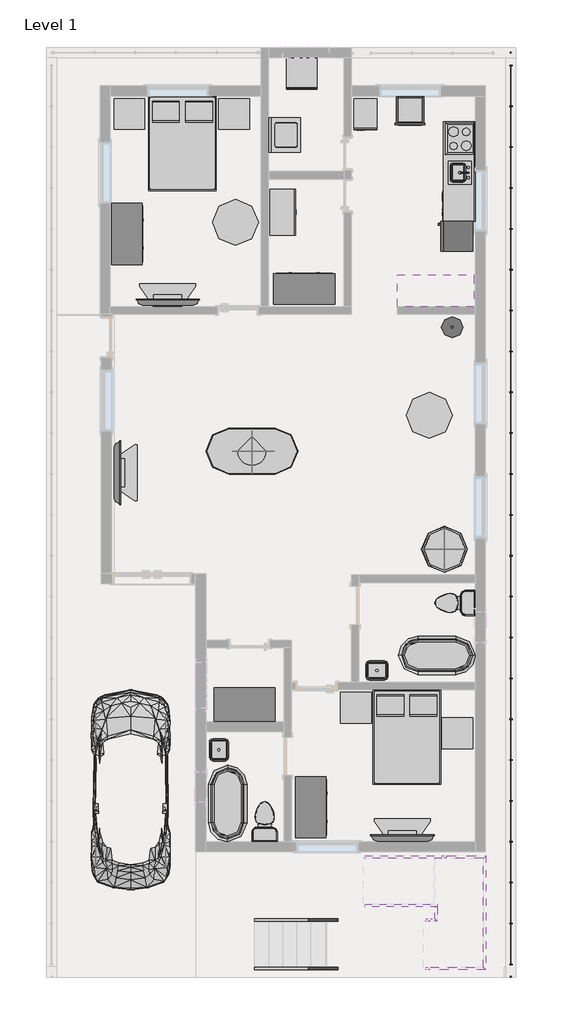
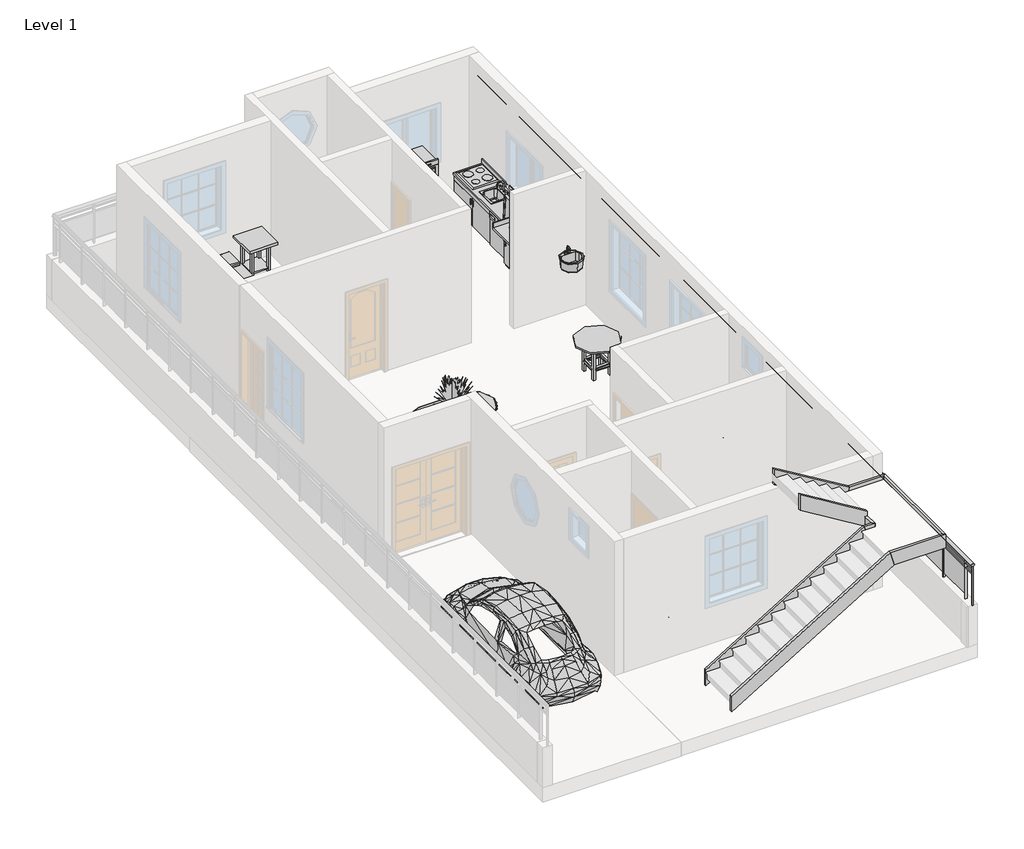
# One storey, part 3 of 3: 23 furniture elements, 9 members, 9 proxies, 8 flow terminals, 2 geographic elements, 1 railing.
# Revit data of these elements (continued)
# Element 34 (IfcFurniture, "Table-Dining Round w Chairs : 36\" Diameter")
#   Phase Created = New Construction
#   Materials on its faces: "Pine", "Laminate, Linen, Matte"
# Element 35 (IfcFurniture, "Table-Ellipse : 72\" x 36\"")
#   Phase Created = New Construction
#   Materials on its faces: "Birch", "Laminate - Black"
# Elements 36, 37, 38, 39 (IfcFurniture, "Table-Night Stand : 24\" x 24\" x 30\"")
#   Phase Created = New Construction
#   Materials on its faces: "Birch", "Laminate, Ivory, Matte"
# Element 40 (IfcFurniture, "Table-Round : 36\" Diameter")
#   Phase Created = New Construction
#   Materials on its faces: "Steel, Chrome Plated", "Birch"
# Element 41 (IfcGeographicElement, "RPC Plant - Tropical : Agave - 1.5'")
#   Phase Created = New Construction
# Element 42 (IfcGeographicElement, "RPC Plant - Tropical : Dagger - 2'")
#   Phase Created = New Construction
# Elements 43, 44, 45, 46, 47, 48, 49, 50, 51 (IfcMember, "Stringer - 2\" Width")
#   Phase Created = New Construction
# Element 52 (IfcRailing, "Glass Panel - Bottom Fill")
#   built-in parameter 1008621 = 3 (stored number, unit not read)
#   Phase Created = New Construction
#   Materials on its faces: "Glass"
# Materials
#   "Plastic, Opaque Black": class "Plastic", colour RGB 0 0 0, transparency 0.7, Description = "Plastic, generic, opaque black", Cost = 0
#   "Steel, Paint Finish, Ivory, Matte": class "Metal", colour RGB 247 247 239, transparency 0, Description = "Steel, paint finish, ivory, matte", Cost = 0
#   "Steel, Chrome Plated": class "Metal", colour RGB 17 17 17, transparency 0, Description = "Chromiuim plated steel", Cost = 0
#   "Steel, Polished": class "Metal", colour RGB 57 57 57, transparency 0, Description = "Polished steel", Cost = 0
#   "Steel, Paint Finish, Ivory, Glossy": class "Metal", colour RGB 247 247 239, transparency 0, Description = "Steel, paint finish, ivory, glossy", Cost = 0
#   "Cabinets": colour RGB 249 249 249, transparency 0
#   "Cabinets - Handles": class "Metal", colour RGB 57 57 57, transparency 0
#   "Metal - Stainless Steel, Polished": class "Metal", colour RGB 216 216 216, transparency 0
#   "Porcelain, Linen": class "Ceramic", colour RGB 249 239 230, transparency 0, Description = "Porcelain, linen", Cost = 0
#   "Laminate, Linen, Matte": class "Plastic", colour RGB 249 239 230, transparency 0, Description = "Plastic Laminate - Linen, Matte", Cost = 0
#   "Porcelain, Ivory": class "Ceramic", colour RGB 247 247 239, transparency 0, Description = "Porcelain, ivory", Cost = 0
#   "Birch": class "Wood", colour RGB 224 178 126, transparency 0, Description = "Betula Alleghaniensis", Cost = 0
#   "Linen, White": class "Textile", colour RGB 247 247 239, transparency 0, Description = "Linen, white", Cost = 0
#   "Laminate - Ivory, Glossy": colour RGB 247 247 239, transparency 0
#   "Laminate, Ivory, Matte": class "Plastic", colour RGB 247 247 239, transparency 0, Description = "Plastic Laminate - Ivory, Matte", Cost = 0
#   "Cherry": class "Wood", colour RGB 226 177 128, transparency 0, Description = "Prunus Serotina", Cost = 0
#   "Melamine - Gray": class "Wood", colour RGB 49 49 49, transparency 0
#   "Glass - Clear, Grey": class "Glass", colour RGB 252 255 255, transparency 0.64
#   "Pine": class "Wood", colour RGB 223 192 134, transparency 0, Description = "Pinus Echinata", Cost = 0
#   "Laminate - Black": colour RGB 0 0 0, transparency 0
#   "Steel": class "Metal", colour RGB 247 247 247, transparency 0, Description = "Steel, mill finish", Cost = 0
#   "Glass": class "Glass", colour RGB 0 128 192, transparency 0.75, Description = "Soda Lime Glass", Cost = 0
#   "Counter Top": class "Wood", colour RGB 226 177 128, transparency 0
#   "TV - Black": colour RGB 49 49 49, transparency 0
#   "TV - Glass": colour RGB 157 157 157, transparency 0.9
#   "TV - Screen": colour RGB 0 0 0, transparency 0
#   "Glass - Shelves": class "Glass", colour RGB 167 167 167, transparency 0.9
